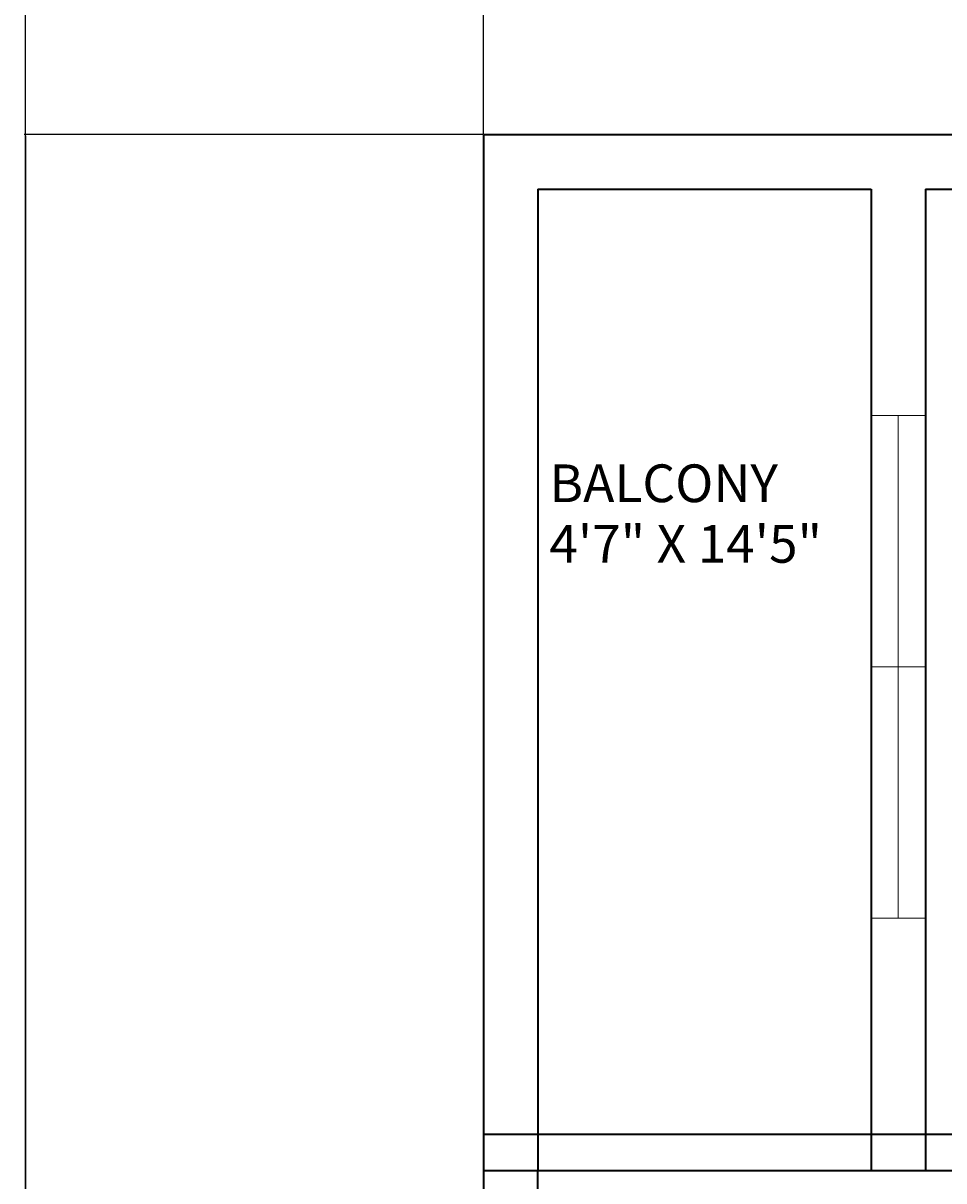
# Model space of a CAD drawing. Units: inches. Extents: x -61 to 1599, y -1316 to 257.
# Tile 32 of 204: x -61 to 91, y -790 to -599. Entities that reach past the tile are written whole.
import ezdxf

# ---------------------------------------------------------------- set-up
doc = ezdxf.new("R2010")
doc.units = ezdxf.units.IN
doc.header["$MEASUREMENT"] = 0
for name, color, linetype, lineweight in [('A-ANNO-DIMS', 2, 'Continuous', 18), ('A-AREA-IDEN', 1, 'Continuous', 18), ('WALLS', 4, 'Continuous', 35), ('WINDOWS', 220, 'Continuous', 18)]:
    doc.layers.add(name, color=color, linetype=linetype, lineweight=lineweight)
doc.styles.get("Standard").update_dxf_attribs({"font": 'arial.ttf'})
doc.dimstyles.get("Standard").update_dxf_attribs({"dimtxt": 0.18, "dimasz": 0.18, "dimexe": 0.18, "dimexo": 0.0625, "dimgap": 0.09, "dimtad": 0, "dimtih": 1, "dimtoh": 1, "dimdec": 0, "dimzin": 0, "dimdsep": 46, "dimlunit": 3, "dimtxsty": 'Standard', "dimcen": 0.09, "dimadec": 0, "dimazin": 0, "dimtfac": 1, "dimtdec": 0, "dimtofl": 0, "dimtmove": 0, "dimatfit": 3, "dimfxl": 1, "dimtolj": 1, "dimtzin": 0, "dimarcsym": 0})

# ---------------------------------------------------------------- blocks, each defined once
blk = doc.blocks.new('WIN-83IN')
for p, q in [((0, 82.94), (9, 82.94)), ((0, 0), (9, 0))]:
    blk.add_line(p, q)
for points in [[(9, 82.94), (4.5, 82.94), (4.5, 41.47), (9, 41.47)], [(4.5, 41.47), (0, 41.47), (0, 0), (4.5, 0)]]:
    blk.add_lwpolyline(points, close=True)
blk = doc.blocks.new('*D687')
at = {"layer": 'A-ANNO-DIMS', "color": 0, "lineweight": -2, "transparency": 16777216}
for p, q in [((289.42, 181.68), (-61.08, 181.68)), ((-60.9, 181.5), (-60.9, -528.95)), ((-60.9, -1239.76), (-60.9, -529.32)), ((319.64, -1239.94), (-61.08, -1239.94))]:
    blk.add_line(p, q, dxfattribs=at)
at = {"layer": 'A-ANNO-DIMS', "color": 0, "transparency": 16777216}
for points in [[(-60.93, 181.5), (-60.87, 181.5), (-60.9, 181.68)], [(-60.93, -1239.76), (-60.87, -1239.76), (-60.9, -1239.94)]]:
    blk.add_solid(points, dxfattribs=at)
at = {"layer": 'DEFPOINTS', "color": 0, "transparency": 16777216}
for p in [(289.48, 181.68), (-60.9, -1239.94), (319.7, -1239.94)]:
    blk.add_point(p, dxfattribs=at)
at = {"layer": 'A-ANNO-DIMS', "color": 0, "transparency": 16777216, "insert": (-60.9, -529.13), "char_height": 0.18, "attachment_point": 5}
blk.add_mtext('\\A1;1421.6', dxfattribs=at)
blk = doc.blocks.new('*D692')
at = {"layer": 'A-ANNO-DIMS', "color": 0, "lineweight": -2, "transparency": 16777216}
for p, q in [((14.64, -441.32), (-61.08, -441.32)), ((-60.9, -441.5), (-60.9, -528.95)), ((-60.9, -616.76), (-60.9, -529.32)), ((14.64, -616.94), (-61.08, -616.94))]:
    blk.add_line(p, q, dxfattribs=at)
at = {"layer": 'A-ANNO-DIMS', "color": 0, "transparency": 16777216}
for points in [[(-60.93, -441.5), (-60.87, -441.5), (-60.9, -441.32)], [(-60.93, -616.76), (-60.87, -616.76), (-60.9, -616.94)]]:
    blk.add_solid(points, dxfattribs=at)
at = {"layer": 'DEFPOINTS', "color": 0, "transparency": 16777216}
for p in [(-60.9, -441.32), (14.7, -441.32), (14.7, -616.94)]:
    blk.add_point(p, dxfattribs=at)
at = {"layer": 'A-ANNO-DIMS', "color": 0, "transparency": 16777216, "insert": (-60.9, -529.13), "char_height": 0.18, "attachment_point": 5}
blk.add_mtext('\\A1;175.62', dxfattribs=at)
blk = doc.blocks.new('*D693')
at = {"layer": 'A-ANNO-DIMS', "color": 0, "lineweight": -2, "transparency": 16777216}
for p, q in [((14.64, -616.94), (-61.08, -616.94)), ((-60.9, -617.12), (-60.9, -916.26)), ((-60.9, -1215.76), (-60.9, -916.63)), ((14.64, -1215.94), (-61.08, -1215.94))]:
    blk.add_line(p, q, dxfattribs=at)
at = {"layer": 'A-ANNO-DIMS', "color": 0, "transparency": 16777216}
for points in [[(-60.93, -617.12), (-60.87, -617.12), (-60.9, -616.94)], [(-60.93, -1215.76), (-60.87, -1215.76), (-60.9, -1215.94)]]:
    blk.add_solid(points, dxfattribs=at)
at = {"layer": 'DEFPOINTS', "color": 0, "transparency": 16777216}
for p in [(-60.9, -616.94), (14.7, -616.94), (14.7, -1215.94)]:
    blk.add_point(p, dxfattribs=at)
at = {"layer": 'A-ANNO-DIMS', "color": 0, "transparency": 16777216, "insert": (-60.9, -916.44), "char_height": 0.18, "attachment_point": 5}
blk.add_mtext('\\A1;599', dxfattribs=at)
blk = doc.blocks.new('*D700')
at = {"layer": 'A-ANNO-DIMS', "color": 0, "lineweight": -2, "transparency": 16777216}
for p, q in [((14.7, -616.88), (14.7, 257.46)), ((14.88, 257.28), (96.77, 257.28)), ((179.57, 257.28), (97.68, 257.28)), ((179.75, -616.88), (179.75, 257.46))]:
    blk.add_line(p, q, dxfattribs=at)
at = {"layer": 'A-ANNO-DIMS', "color": 0, "transparency": 16777216}
for points in [[(14.88, 257.31), (14.88, 257.25), (14.7, 257.28)], [(179.57, 257.31), (179.57, 257.25), (179.75, 257.28)]]:
    blk.add_solid(points, dxfattribs=at)
at = {"layer": 'DEFPOINTS', "color": 0, "transparency": 16777216}
for p in [(179.75, 257.28), (14.7, -616.94), (179.75, -616.94)]:
    blk.add_point(p, dxfattribs=at)
at = {"layer": 'A-ANNO-DIMS', "color": 0, "transparency": 16777216, "insert": (97.23, 257.28), "char_height": 0.18, "attachment_point": 5}
blk.add_mtext('\\A1;165.05', dxfattribs=at)

msp = doc.modelspace()

# ---------------------------------------------------------------- linework, layer by layer
at = {"layer": 'WALLS'}
for p, q in [((14.7028, -616.9446), (14.7028, -1215.9446)), ((544.7028, -616.9446), (14.7028, -616.9446)), ((23.7028, -625.9446), (23.7028, -787.9446)), ((23.7028, -625.9446), (78.7028, -625.9446)), ((78.7028, -625.9446), (78.7028, -787.9446)), ((87.7028, -625.9446), (87.7028, -787.9446)), ((87.7028, -625.9446), (231.7028, -625.9446)), ((14.7028, -781.9446), (237.7028, -781.9446)), ((14.7028, -787.9446), (237.7028, -787.9446)), ((23.7028, -943.9446), (23.7028, -787.9446))]:
    msp.add_line(p, q, dxfattribs=at)

# ---------------------------------------------------------------- block references
at = {"layer": 'WINDOWS'}
msp.add_blockref('WIN-83IN', (78.703, -746.2567), dxfattribs=at)

# ---------------------------------------------------------------- texts
at = {"layer": 'A-AREA-IDEN'}
for s, height, p in [('BALCONY', 6.22364, (25.5954, -677.6027)), ('4\'7" X 14\'5"', 6.223643, (25.5954, -687.6005))]:
    msp.add_text(s, height=height, dxfattribs=at).set_placement(p)

# ---------------------------------------------------------------- dimensions: what is measured, and where the dimension line sits
at = {"layer": 'A-ANNO-DIMS'}
dim = msp.add_linear_dim(base=(179.7521, 257.2771), p1=(14.7028, -616.9446), p2=(179.7521, -616.9446), dimstyle='Standard', override={"dimdec": 2, "dimlfac": 1, "dimrnd": 0, "dimzin": 0, "dimdsep": 46, "dimlunit": 2}, dxfattribs=at)
dim.commit()
dim.dimension.update_dxf_attribs({"geometry": '*D700', "text_midpoint": (97.2274, 257.2771)})
for base, p1, p2, override, picture, middle in [((-60.8972, -1239.9446), (289.4807, 181.6771), (319.7028, -1239.9446), {"dimdec": 1, "dimlfac": 1, "dimrnd": 0, "dimzin": 0, "dimdsep": 46, "dimlunit": 2}, '*D687', (-60.8972, -529.1337)), ((-60.8972, -441.3229), (14.7028, -616.9446), (14.7028, -441.3229), {"dimdec": 2, "dimlfac": 1, "dimrnd": 0, "dimzin": 0, "dimdsep": 46, "dimlunit": 2}, '*D692', (-60.8972, -529.1337)), ((-60.8972, -616.9446), (14.7028, -1215.9446), (14.7028, -616.9446), {"dimdec": 0, "dimlfac": 1, "dimrnd": 0, "dimzin": 0, "dimdsep": 46, "dimlunit": 2}, '*D693', (-60.8972, -916.4446))]:
    dim = msp.add_linear_dim(base=base, p1=p1, p2=p2, angle=90, dimstyle='Standard', override=override, dxfattribs=at)
    dim.commit()
    dim.dimension.update_dxf_attribs({"geometry": picture, "text_midpoint": middle})

doc.saveas('drawing.dxf')
